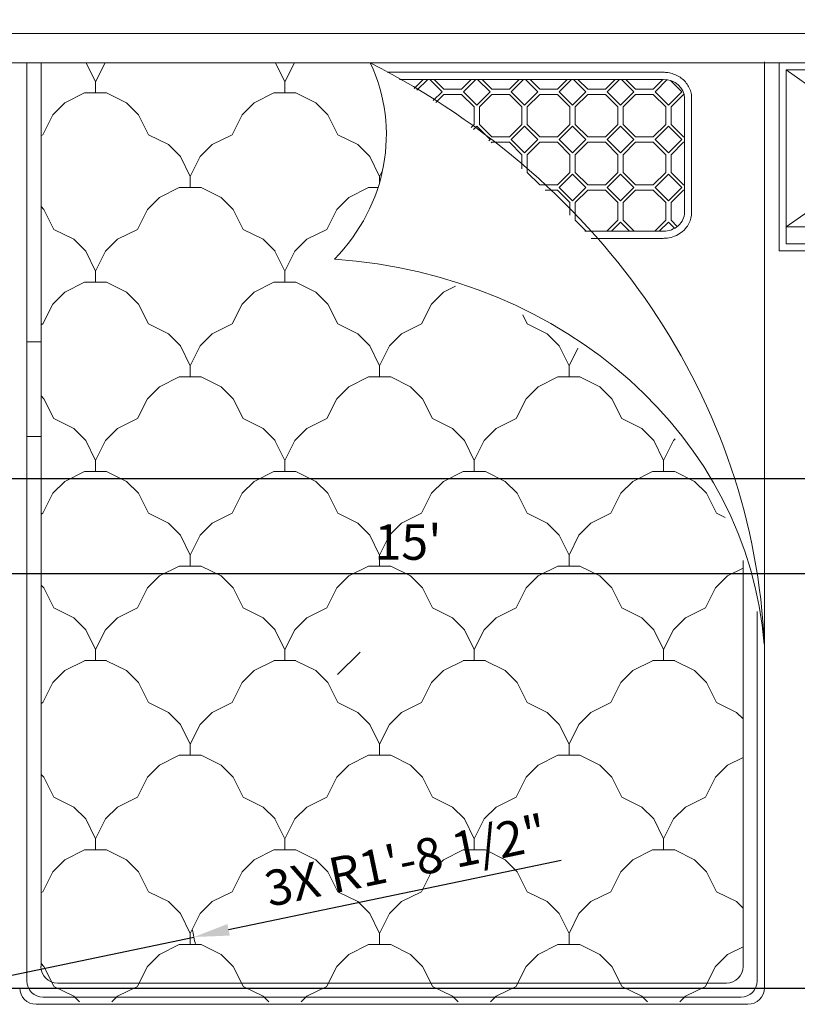
# Model space of a CAD drawing. Units: inches. Extents: x 2025 to 2528, y 1525 to 2336.
# Tile 12 of 18: x 2138 to 2192, y 2209 to 2278. Entities that reach past the tile are written whole.
import ezdxf

# ---------------------------------------------------------------- set-up
doc = ezdxf.new("R2010")
doc.units = ezdxf.units.IN
doc.layers.add('A-ANNO-DIMS', color=2, linetype='Continuous', lineweight=18)
doc.layers.add('A-FURN', color=8, linetype='Continuous', lineweight=18)
doc.styles.get("Standard").update_dxf_attribs({"font": 'arial.ttf'})
doc.dimstyles.new('Copy of ISO-25', dxfattribs={"dimtxt": 2.5, "dimasz": 2.5, "dimexe": 1.25, "dimexo": 0.625, "dimtad": 1, "dimdec": 1, "dimlunit": 4, "dimtxsty": 'Standard', "dimcen": 2.5, "dimadec": 0, "dimazin": 0, "dimtfac": 1, "dimtdec": 1, "dimtmove": 0, "dimatfit": 3, "dimfxl": 1, "dimarcsym": 0})

# ---------------------------------------------------------------- blocks, each defined once
blk = doc.blocks.new('*D6')
at = {"layer": 'A-ANNO-DIMS', "color": 0, "lineweight": -2, "transparency": 16777216}
for p, q in [((2075.013, 2282.787), (2075.013, 2237.927)), ((2255.013, 2282.787), (2255.013, 2237.927)), ((2077.513, 2239.177), (2252.513, 2239.177))]:
    blk.add_line(p, q, dxfattribs=at)
at = {"layer": 'A-ANNO-DIMS', "color": 0, "transparency": 16777216}
for points in [[(2077.513, 2239.594), (2077.513, 2238.761), (2075.013, 2239.177)], [(2252.513, 2239.594), (2252.513, 2238.761), (2255.013, 2239.177)]]:
    blk.add_solid(points, dxfattribs=at)
at = {"layer": 'Defpoints', "color": 0, "transparency": 16777216}
for p in [(2075.013, 2283.412), (2255.013, 2283.412), (2255.013, 2239.177)]:
    blk.add_point(p, dxfattribs=at)
at = {"layer": 'A-ANNO-DIMS', "color": 0, "transparency": 16777216, "insert": (2165.013, 2241.079), "char_height": 2.5, "attachment_point": 5}
blk.add_mtext("15'", dxfattribs=at)
blk = doc.blocks.new('A$C029D5C69')
for p, q in [((2.2315, 2.0693), (0.4164, 2.0693)), ((0.4164, 2.0066), (2.2315, 2.0066)), ((0.5403, 0.0502), (0.5403, 2.0066)), ((0.5706, 0.0805), (0.5706, 2.0066)), ((0.6869, 1.966), (0.6666, 2.0066)), ((0.7072, 2.0066), (0.6869, 1.966)), ((1.0902, 1.966), (1.0699, 2.0066)), ((1.1106, 2.0066), (1.0902, 1.966)), ((2.1114, 2.0087), (2.1114, 0.0351)), ((2.6479, 2.0066), (2.1429, 2.0066)), ((2.1429, 2.0066), (2.1429, 1.606)), ((1.8954, 1.9865), (1.3081, 1.9865)), ((2.6328, 1.9915), (2.158, 1.9915)), ((2.158, 1.9915), (2.158, 1.6211)), ((0.6869, 1.9425), (0.6869, 1.966)), ((0.6869, 1.9425), (0.6869, 1.966)), ((1.0902, 1.9425), (1.0902, 1.966)), ((1.0902, 1.9425), (1.0902, 1.966)), ((1.8954, 1.9713), (1.3339, 1.9713)), ((1.3849, 1.9713), (1.3656, 1.952)), ((1.3945, 1.9713), (1.3714, 1.9483)), ((1.4249, 1.945), (1.3986, 1.9713)), ((1.4288, 1.9507), (1.4081, 1.9713)), ((1.487, 1.9713), (1.4664, 1.9507)), ((1.4966, 1.9713), (1.4703, 1.945)), ((1.527, 1.945), (1.5007, 1.9713)), ((1.5309, 1.9507), (1.5102, 1.9713)), ((1.5891, 1.9713), (1.5685, 1.9507)), ((1.5987, 1.9713), (1.5724, 1.945)), ((1.6291, 1.945), (1.6028, 1.9713)), ((1.633, 1.9507), (1.6123, 1.9713)), ((1.6912, 1.9713), (1.6706, 1.9507)), ((1.7008, 1.9713), (1.6745, 1.945)), ((1.7312, 1.945), (1.7049, 1.9713)), ((1.7351, 1.9507), (1.7144, 1.9713)), ((1.7933, 1.9713), (1.7727, 1.9507)), ((1.8029, 1.9713), (1.7766, 1.945)), ((1.8333, 1.945), (1.807, 1.9713)), ((1.8372, 1.9507), (1.8165, 1.9713)), ((1.8954, 1.9713), (1.8748, 1.9507)), ((1.9043, 1.9707), (1.8787, 1.945)), ((1.9354, 1.945), (1.9114, 1.969)), ((0.6634, 1.9425), (0.621, 1.9213)), ((0.6634, 1.9425), (0.621, 1.9213)), ((0.6869, 1.9425), (0.6634, 1.9425)), ((0.6869, 1.9425), (0.7104, 1.9425)), ((0.7528, 1.9213), (0.7104, 1.9425)), ((0.7528, 1.9213), (0.7104, 1.9425)), ((1.0668, 1.9425), (1.0244, 1.9213)), ((1.0668, 1.9425), (1.0244, 1.9213)), ((1.0902, 1.9425), (1.0668, 1.9425)), ((1.0902, 1.9425), (1.1137, 1.9425)), ((1.1561, 1.9213), (1.1137, 1.9425)), ((1.1561, 1.9213), (1.1137, 1.9425)), ((1.4249, 1.945), (1.4059, 1.926)), ((1.4288, 1.9394), (1.4116, 1.9222)), ((1.4476, 1.9507), (1.4288, 1.9507)), ((1.4288, 1.9393), (1.4476, 1.9393)), ((1.4476, 1.9507), (1.4664, 1.9507)), ((1.4664, 1.9393), (1.4476, 1.9393)), ((1.493, 1.9128), (1.4664, 1.9394)), ((1.4986, 1.9167), (1.4703, 1.945)), ((1.527, 1.945), (1.4986, 1.9167)), ((1.5309, 1.9394), (1.5043, 1.9128)), ((1.5497, 1.9507), (1.5309, 1.9507)), ((1.5309, 1.9393), (1.5497, 1.9393)), ((1.5497, 1.9507), (1.5685, 1.9507)), ((1.5685, 1.9393), (1.5497, 1.9393)), ((1.595, 1.9128), (1.5685, 1.9394)), ((1.6007, 1.9167), (1.5724, 1.945)), ((1.6291, 1.945), (1.6007, 1.9167)), ((1.633, 1.9394), (1.6064, 1.9128)), ((1.6518, 1.9507), (1.633, 1.9507)), ((1.633, 1.9393), (1.6518, 1.9393)), ((1.6518, 1.9507), (1.6706, 1.9507)), ((1.6706, 1.9393), (1.6518, 1.9393)), ((1.6971, 1.9128), (1.6706, 1.9394)), ((1.7028, 1.9167), (1.6745, 1.945)), ((1.7312, 1.945), (1.7028, 1.9167)), ((1.7351, 1.9394), (1.7085, 1.9128)), ((1.7539, 1.9507), (1.7351, 1.9507)), ((1.7351, 1.9393), (1.7539, 1.9393)), ((1.7539, 1.9507), (1.7727, 1.9507)), ((1.7727, 1.9393), (1.7539, 1.9393)), ((1.7992, 1.9128), (1.7727, 1.9394)), ((1.8049, 1.9167), (1.7766, 1.945)), ((1.8333, 1.945), (1.8049, 1.9167)), ((1.8372, 1.9394), (1.8106, 1.9128)), ((1.856, 1.9507), (1.8372, 1.9507)), ((1.8372, 1.9393), (1.856, 1.9393)), ((1.856, 1.9507), (1.8748, 1.9507)), ((1.8748, 1.9393), (1.856, 1.9393)), ((1.9013, 1.9128), (1.8748, 1.9394)), ((1.907, 1.9167), (1.8787, 1.945)), ((1.9354, 1.945), (1.907, 1.9167)), ((1.9393, 1.9394), (1.9127, 1.9128)), ((1.9393, 1.9393), (1.9404, 1.9393)), ((1.9414, 1.688), (1.9414, 1.931)), ((1.9565, 1.688), (1.9565, 1.931)), ((0.621, 1.9213), (0.5955, 1.8958)), ((0.7783, 1.8958), (0.7528, 1.9213)), ((1.0243, 1.9213), (0.9988, 1.8958)), ((1.1816, 1.8958), (1.1561, 1.9213)), ((1.493, 1.8752), (1.493, 1.9128)), ((1.5043, 1.8752), (1.5043, 1.9128)), ((1.595, 1.8752), (1.595, 1.9128)), ((1.6064, 1.8752), (1.6064, 1.9128)), ((1.6971, 1.8752), (1.6971, 1.9128)), ((1.7085, 1.8752), (1.7085, 1.9128)), ((1.7992, 1.8752), (1.7992, 1.9128)), ((1.8106, 1.8752), (1.8106, 1.9128)), ((1.9013, 1.8752), (1.9013, 1.9128)), ((1.9127, 1.8752), (1.9127, 1.9128)), ((0.5955, 1.8958), (0.5743, 1.8534)), ((0.7995, 1.8534), (0.7783, 1.8958)), ((0.9989, 1.8958), (0.9777, 1.8534)), ((1.2028, 1.8534), (1.1816, 1.8958)), ((1.493, 1.8752), (1.4867, 1.869)), ((1.4986, 1.8713), (1.4922, 1.8648)), ((1.527, 1.8429), (1.4986, 1.8713)), ((1.5309, 1.8486), (1.5043, 1.8752)), ((1.595, 1.8752), (1.5685, 1.8486)), ((1.6007, 1.8713), (1.5724, 1.8429)), ((1.6291, 1.8429), (1.6007, 1.8713)), ((1.633, 1.8486), (1.6064, 1.8752)), ((1.6971, 1.8752), (1.6706, 1.8486)), ((1.7028, 1.8713), (1.6745, 1.8429)), ((1.7312, 1.8429), (1.7028, 1.8713)), ((1.7351, 1.8486), (1.7085, 1.8752)), ((1.7992, 1.8752), (1.7727, 1.8486)), ((1.8049, 1.8713), (1.7766, 1.8429)), ((1.8333, 1.8429), (1.8049, 1.8713)), ((1.8372, 1.8486), (1.8106, 1.8752)), ((1.9013, 1.8752), (1.8748, 1.8486)), ((1.907, 1.8713), (1.8787, 1.8429)), ((1.9354, 1.8429), (1.907, 1.8713)), ((1.9393, 1.8486), (1.9127, 1.8752)), ((0.5743, 1.8534), (0.5706, 1.8515)), ((0.5743, 1.8534), (0.5706, 1.8515)), ((0.8419, 1.8322), (0.7995, 1.8534)), ((0.8419, 1.8322), (0.7995, 1.8534)), ((0.9777, 1.8534), (0.9353, 1.8322)), ((0.9777, 1.8534), (0.9353, 1.8322)), ((1.2452, 1.8322), (1.2028, 1.8534)), ((1.2452, 1.8322), (1.2028, 1.8534)), ((1.5497, 1.8486), (1.5309, 1.8486)), ((1.5497, 1.8486), (1.5685, 1.8486)), ((1.6518, 1.8486), (1.633, 1.8486)), ((1.6518, 1.8486), (1.6706, 1.8486)), ((1.7539, 1.8486), (1.7351, 1.8486)), ((1.7539, 1.8486), (1.7727, 1.8486)), ((1.856, 1.8486), (1.8372, 1.8486)), ((1.856, 1.8486), (1.8748, 1.8486)), ((1.9414, 1.8486), (1.9393, 1.8486)), ((0.8674, 1.8067), (0.8419, 1.8322)), ((0.9352, 1.8322), (0.9097, 1.8067)), ((1.2707, 1.8067), (1.2452, 1.8322)), ((1.527, 1.8429), (1.5242, 1.8401)), ((1.5309, 1.8373), (1.5295, 1.8359)), ((1.5309, 1.8373), (1.5497, 1.8373)), ((1.5685, 1.8373), (1.5497, 1.8373)), ((1.595, 1.8107), (1.5685, 1.8373)), ((1.6007, 1.8146), (1.5724, 1.8429)), ((1.6291, 1.8429), (1.6007, 1.8146)), ((1.633, 1.8373), (1.6064, 1.8107)), ((1.633, 1.8373), (1.6518, 1.8373)), ((1.6706, 1.8373), (1.6518, 1.8373)), ((1.6971, 1.8107), (1.6706, 1.8373)), ((1.7028, 1.8146), (1.6745, 1.8429)), ((1.7312, 1.8429), (1.7028, 1.8146)), ((1.7351, 1.8373), (1.7085, 1.8107)), ((1.7351, 1.8373), (1.7539, 1.8373)), ((1.7727, 1.8373), (1.7539, 1.8373)), ((1.7992, 1.8107), (1.7727, 1.8373)), ((1.8049, 1.8146), (1.7766, 1.8429)), ((1.8333, 1.8429), (1.8049, 1.8146)), ((1.8372, 1.8373), (1.8106, 1.8107)), ((1.8372, 1.8373), (1.856, 1.8373)), ((1.8748, 1.8373), (1.856, 1.8373)), ((1.9013, 1.8107), (1.8748, 1.8373)), ((1.907, 1.8146), (1.8787, 1.8429)), ((1.9354, 1.8429), (1.907, 1.8146)), ((1.9393, 1.8373), (1.9127, 1.8107)), ((1.9393, 1.8373), (1.9414, 1.8373)), ((0.8886, 1.7643), (0.8674, 1.8067)), ((0.9098, 1.8067), (0.8886, 1.7643)), ((1.2919, 1.7643), (1.2707, 1.8067)), ((1.595, 1.7806), (1.595, 1.8107)), ((1.6064, 1.7731), (1.6064, 1.8107)), ((1.6971, 1.7731), (1.6971, 1.8107)), ((1.7085, 1.7731), (1.7085, 1.8107)), ((1.7992, 1.7731), (1.7992, 1.8107)), ((1.8106, 1.7731), (1.8106, 1.8107)), ((1.9013, 1.7731), (1.9013, 1.8107)), ((1.9127, 1.7731), (1.9127, 1.8107)), ((0.8886, 1.7408), (0.8886, 1.7643)), ((1.2981, 1.7768), (1.2919, 1.7643)), ((1.2919, 1.7519), (1.2919, 1.7643)), ((1.633, 1.7465), (1.6064, 1.7731)), ((1.6971, 1.7731), (1.6706, 1.7465)), ((1.7028, 1.7692), (1.6745, 1.7408)), ((1.7312, 1.7408), (1.7028, 1.7692)), ((1.7351, 1.7465), (1.7085, 1.7731)), ((1.7992, 1.7731), (1.7727, 1.7465)), ((1.8049, 1.7692), (1.7766, 1.7408)), ((1.8333, 1.7408), (1.8049, 1.7692)), ((1.8372, 1.7465), (1.8106, 1.7731)), ((1.9013, 1.7731), (1.8748, 1.7465)), ((1.907, 1.7692), (1.8787, 1.7408)), ((1.9354, 1.7408), (1.907, 1.7692)), ((1.9393, 1.7465), (1.9127, 1.7731)), ((1.6518, 1.7465), (1.633, 1.7465)), ((1.6518, 1.7465), (1.6706, 1.7465)), ((1.7539, 1.7465), (1.7351, 1.7465)), ((1.7539, 1.7465), (1.7727, 1.7465)), ((1.856, 1.7465), (1.8372, 1.7465)), ((1.856, 1.7465), (1.8748, 1.7465)), ((1.9414, 1.7465), (1.9393, 1.7465)), ((0.8651, 1.7408), (0.8227, 1.7196)), ((0.8651, 1.7408), (0.8227, 1.7196)), ((0.912, 1.7408), (0.8651, 1.7408)), ((0.9544, 1.7196), (0.912, 1.7408)), ((0.9544, 1.7196), (0.912, 1.7408)), ((1.2684, 1.7408), (1.226, 1.7196)), ((1.2684, 1.7408), (1.226, 1.7196)), ((1.2885, 1.7408), (1.2684, 1.7408)), ((1.6443, 1.7352), (1.6518, 1.7352)), ((1.6706, 1.7352), (1.6518, 1.7352)), ((1.6971, 1.7086), (1.6706, 1.7352)), ((1.7028, 1.7125), (1.6745, 1.7408)), ((1.7312, 1.7408), (1.7028, 1.7125)), ((1.7351, 1.7352), (1.7085, 1.7086)), ((1.7351, 1.7352), (1.7539, 1.7352)), ((1.7727, 1.7352), (1.7539, 1.7352)), ((1.7992, 1.7086), (1.7727, 1.7352)), ((1.8049, 1.7125), (1.7766, 1.7408)), ((1.8333, 1.7408), (1.8049, 1.7125)), ((1.8372, 1.7352), (1.8106, 1.7086)), ((1.8372, 1.7352), (1.856, 1.7352)), ((1.8748, 1.7352), (1.856, 1.7352)), ((1.9013, 1.7086), (1.8748, 1.7352)), ((1.907, 1.7125), (1.8787, 1.7408)), ((1.9354, 1.7408), (1.907, 1.7125)), ((1.9393, 1.7352), (1.9127, 1.7086)), ((1.9393, 1.7352), (1.9414, 1.7352)), ((0.5766, 1.6941), (0.5706, 1.7002)), ((0.8227, 1.7196), (0.7972, 1.6941)), ((0.98, 1.6941), (0.9545, 1.7196)), ((1.226, 1.7196), (1.2005, 1.6941)), ((1.6971, 1.682), (1.6971, 1.7086)), ((1.7085, 1.671), (1.7085, 1.7086)), ((1.7992, 1.671), (1.7992, 1.7086)), ((1.8106, 1.671), (1.8106, 1.7086)), ((1.9013, 1.671), (1.9013, 1.7086)), ((1.9127, 1.671), (1.9127, 1.7086)), ((0.5978, 1.6517), (0.5766, 1.6941)), ((0.7972, 1.6941), (0.776, 1.6517)), ((1.0011, 1.6517), (0.9799, 1.6941)), ((1.2005, 1.6941), (1.1793, 1.6517)), ((1.7318, 1.6477), (1.7085, 1.671)), ((1.7992, 1.671), (1.7759, 1.6477)), ((1.8049, 1.6671), (1.7855, 1.6477)), ((1.8244, 1.6477), (1.8049, 1.6671)), ((1.8339, 1.6477), (1.8106, 1.671)), ((1.9013, 1.671), (1.878, 1.6477)), ((1.907, 1.6671), (1.8876, 1.6477)), ((1.9202, 1.6539), (1.907, 1.6671)), ((1.926, 1.6577), (1.9127, 1.671)), ((0.6402, 1.6305), (0.5978, 1.6517)), ((0.6402, 1.6305), (0.5978, 1.6517)), ((0.776, 1.6517), (0.7336, 1.6305)), ((0.776, 1.6517), (0.7336, 1.6305)), ((1.0435, 1.6305), (1.0011, 1.6517)), ((1.0435, 1.6305), (1.0011, 1.6517)), ((1.1793, 1.6517), (1.1369, 1.6305)), ((1.1793, 1.6517), (1.1369, 1.6305)), ((1.8961, 1.6477), (1.7289, 1.6477)), ((0.6657, 1.605), (0.6402, 1.6305)), ((0.7336, 1.6305), (0.7081, 1.605)), ((1.0691, 1.605), (1.0436, 1.6305)), ((1.1369, 1.6305), (1.1114, 1.605)), ((1.8961, 1.6325), (1.7422, 1.6325)), ((2.158, 1.6211), (2.6328, 1.6211)), ((0.6869, 1.5626), (0.6657, 1.605)), ((0.7081, 1.605), (0.6869, 1.5626)), ((1.0902, 1.5626), (1.069, 1.605)), ((1.1114, 1.605), (1.0902, 1.5626)), ((2.1429, 1.606), (2.6479, 1.606)), ((0.6869, 1.5392), (0.6869, 1.5626)), ((0.6869, 1.5392), (0.6869, 1.5626)), ((1.0902, 1.5392), (1.0902, 1.5626)), ((1.0902, 1.5392), (1.0902, 1.5626)), ((0.6634, 1.5391), (0.621, 1.5179)), ((0.6634, 1.5391), (0.621, 1.5179)), ((0.6869, 1.5392), (0.6634, 1.5392)), ((0.6869, 1.5392), (0.7104, 1.5392)), ((0.7528, 1.5179), (0.7104, 1.5391)), ((0.7528, 1.5179), (0.7104, 1.5391)), ((1.0668, 1.5391), (1.0244, 1.5179)), ((1.0668, 1.5391), (1.0244, 1.5179)), ((1.0902, 1.5392), (1.0668, 1.5392)), ((1.0902, 1.5392), (1.1137, 1.5392)), ((1.1561, 1.5179), (1.1137, 1.5391)), ((1.1561, 1.5179), (1.1137, 1.5391)), ((0.621, 1.5179), (0.5955, 1.4924)), ((0.7783, 1.4924), (0.7528, 1.5179)), ((1.0243, 1.5179), (0.9988, 1.4924)), ((1.1816, 1.4924), (1.1561, 1.5179)), ((1.4277, 1.5179), (1.4022, 1.4924)), ((1.4534, 1.5308), (1.4277, 1.5179)), ((1.4534, 1.5308), (1.4277, 1.5179)), ((0.5955, 1.4925), (0.5743, 1.4501)), ((0.7995, 1.4501), (0.7783, 1.4925)), ((0.9989, 1.4925), (0.9777, 1.4501)), ((1.2028, 1.4501), (1.1816, 1.4925)), ((1.4022, 1.4925), (1.381, 1.4501)), ((1.6062, 1.4501), (1.5966, 1.4692)), ((0.5743, 1.45), (0.5706, 1.4481)), ((0.5743, 1.45), (0.5706, 1.4481)), ((0.8419, 1.4288), (0.7995, 1.45)), ((0.8419, 1.4288), (0.7995, 1.45)), ((0.9777, 1.45), (0.9353, 1.4288)), ((0.9777, 1.45), (0.9353, 1.4288)), ((1.2452, 1.4288), (1.2028, 1.45)), ((1.2452, 1.4288), (1.2028, 1.45)), ((1.381, 1.45), (1.3386, 1.4288)), ((1.381, 1.45), (1.3386, 1.4288)), ((1.6486, 1.4288), (1.6062, 1.45)), ((1.6486, 1.4288), (1.6062, 1.45)), ((0.8674, 1.4033), (0.8419, 1.4288)), ((0.9352, 1.4288), (0.9097, 1.4033)), ((1.2707, 1.4033), (1.2452, 1.4288)), ((1.3386, 1.4288), (1.3131, 1.4033)), ((1.6741, 1.4033), (1.6486, 1.4288)), ((0.5403, 1.4117), (0.5706, 1.4117)), ((0.8886, 1.361), (0.8674, 1.4034)), ((0.9098, 1.4034), (0.8886, 1.361)), ((1.2919, 1.361), (1.2707, 1.4034)), ((1.3131, 1.4034), (1.2919, 1.361)), ((1.6953, 1.361), (1.6741, 1.4034)), ((1.714, 1.3984), (1.6953, 1.361)), ((0.8886, 1.3375), (0.8886, 1.3609)), ((1.2919, 1.3375), (1.2919, 1.3609)), ((1.6953, 1.3375), (1.6953, 1.3609)), ((0.8651, 1.3374), (0.8227, 1.3162)), ((0.8651, 1.3374), (0.8227, 1.3162)), ((0.912, 1.3375), (0.8651, 1.3375)), ((0.9544, 1.3162), (0.912, 1.3374)), ((0.9544, 1.3162), (0.912, 1.3374)), ((1.2684, 1.3374), (1.226, 1.3162)), ((1.2684, 1.3374), (1.226, 1.3162)), ((1.3154, 1.3375), (1.2684, 1.3375)), ((1.3578, 1.3162), (1.3154, 1.3374)), ((1.3578, 1.3162), (1.3154, 1.3374)), ((1.6718, 1.3374), (1.6294, 1.3162)), ((1.6718, 1.3374), (1.6294, 1.3162)), ((1.7187, 1.3375), (1.6718, 1.3375)), ((1.7611, 1.3162), (1.7187, 1.3374)), ((1.7611, 1.3162), (1.7187, 1.3374)), ((0.8227, 1.3163), (0.7972, 1.2908)), ((0.98, 1.2908), (0.9545, 1.3163)), ((1.226, 1.3163), (1.2005, 1.2908)), ((1.3833, 1.2908), (1.3578, 1.3163)), ((1.6294, 1.3163), (1.6039, 1.2908)), ((1.7867, 1.2908), (1.7611, 1.3163)), ((0.5766, 1.2908), (0.5706, 1.2968)), ((0.5978, 1.2484), (0.5766, 1.2908)), ((0.7972, 1.2908), (0.776, 1.2484)), ((1.0011, 1.2484), (0.9799, 1.2908)), ((1.2005, 1.2908), (1.1793, 1.2484)), ((1.4045, 1.2484), (1.3833, 1.2908)), ((1.6039, 1.2908), (1.5827, 1.2484)), ((1.8078, 1.2484), (1.7866, 1.2908)), ((0.6402, 1.2271), (0.5978, 1.2483)), ((0.6402, 1.2271), (0.5978, 1.2483)), ((0.776, 1.2483), (0.7336, 1.2271)), ((0.776, 1.2483), (0.7336, 1.2271)), ((1.0435, 1.2271), (1.0011, 1.2483)), ((1.0435, 1.2271), (1.0011, 1.2483)), ((1.1793, 1.2483), (1.1369, 1.2271)), ((1.1793, 1.2483), (1.1369, 1.2271)), ((1.4469, 1.2271), (1.4045, 1.2483)), ((1.4469, 1.2271), (1.4045, 1.2483)), ((1.5827, 1.2483), (1.5403, 1.2271)), ((1.5827, 1.2483), (1.5403, 1.2271)), ((1.8502, 1.2271), (1.8078, 1.2483)), ((1.8502, 1.2271), (1.8078, 1.2483)), ((0.6657, 1.2017), (0.6402, 1.2272)), ((0.7336, 1.2272), (0.7081, 1.2017)), ((1.0691, 1.2017), (1.0436, 1.2272)), ((1.1369, 1.2272), (1.1114, 1.2017)), ((1.4724, 1.2017), (1.4469, 1.2272)), ((1.5403, 1.2272), (1.5148, 1.2017)), ((1.8758, 1.2017), (1.8503, 1.2272)), ((0.5403, 1.21), (0.5706, 1.21)), ((0.6869, 1.1593), (0.6657, 1.2017)), ((0.7081, 1.2017), (0.6869, 1.1593)), ((1.0902, 1.1593), (1.069, 1.2017)), ((1.1114, 1.2017), (1.0902, 1.1593)), ((1.4936, 1.1593), (1.4724, 1.2017)), ((1.5148, 1.2017), (1.4936, 1.1593)), ((1.8969, 1.1593), (1.8757, 1.2017)), ((1.9181, 1.2017), (1.8969, 1.1593)), ((1.9215, 1.2051), (1.9181, 1.2017)), ((0.6869, 1.1358), (0.6869, 1.1593)), ((0.6869, 1.1358), (0.6869, 1.1593)), ((1.0902, 1.1358), (1.0902, 1.1593)), ((1.0902, 1.1358), (1.0902, 1.1593)), ((1.4936, 1.1358), (1.4936, 1.1593)), ((1.4936, 1.1358), (1.4936, 1.1593)), ((1.8969, 1.1358), (1.8969, 1.1593)), ((1.8969, 1.1358), (1.8969, 1.1593)), ((0.6634, 1.1358), (0.621, 1.1146)), ((0.6634, 1.1358), (0.621, 1.1146)), ((0.6869, 1.1358), (0.6634, 1.1358)), ((0.6869, 1.1358), (0.7104, 1.1358)), ((0.7528, 1.1146), (0.7104, 1.1358)), ((0.7528, 1.1146), (0.7104, 1.1358)), ((1.0668, 1.1358), (1.0244, 1.1146)), ((1.0668, 1.1358), (1.0244, 1.1146)), ((1.0902, 1.1358), (1.0668, 1.1358)), ((1.0902, 1.1358), (1.1137, 1.1358)), ((1.1561, 1.1146), (1.1137, 1.1358)), ((1.1561, 1.1146), (1.1137, 1.1358)), ((1.4701, 1.1358), (1.4277, 1.1146)), ((1.4701, 1.1358), (1.4277, 1.1146)), ((1.4936, 1.1358), (1.4701, 1.1358)), ((1.4936, 1.1358), (1.5171, 1.1358)), ((1.5595, 1.1146), (1.5171, 1.1358)), ((1.5595, 1.1146), (1.5171, 1.1358)), ((1.8735, 1.1358), (1.8311, 1.1146)), ((1.8735, 1.1358), (1.8311, 1.1146)), ((1.8969, 1.1358), (1.8735, 1.1358)), ((1.8969, 1.1358), (1.9204, 1.1358)), ((1.9628, 1.1146), (1.9204, 1.1358)), ((1.9628, 1.1146), (1.9204, 1.1358)), ((0.621, 1.1146), (0.5955, 1.0891)), ((0.7783, 1.0891), (0.7528, 1.1146)), ((1.0243, 1.1146), (0.9988, 1.0891)), ((1.1816, 1.0891), (1.1561, 1.1146)), ((1.4277, 1.1146), (1.4022, 1.0891)), ((1.585, 1.0891), (1.5595, 1.1146)), ((1.831, 1.1146), (1.8055, 1.0891)), ((1.9883, 1.0891), (1.9628, 1.1146)), ((0.5955, 1.0891), (0.5743, 1.0467)), ((0.7995, 1.0467), (0.7783, 1.0891)), ((0.9989, 1.0891), (0.9777, 1.0467)), ((1.2028, 1.0467), (1.1816, 1.0891)), ((1.4022, 1.0891), (1.381, 1.0467)), ((1.6062, 1.0467), (1.585, 1.0891)), ((1.8056, 1.0891), (1.7844, 1.0467)), ((2.0095, 1.0467), (1.9883, 1.0891)), ((0.5743, 1.0467), (0.5706, 1.0448)), ((0.5743, 1.0467), (0.5706, 1.0448)), ((0.8419, 1.0255), (0.7995, 1.0467)), ((0.8419, 1.0255), (0.7995, 1.0467)), ((0.9777, 1.0467), (0.9353, 1.0255)), ((0.9777, 1.0467), (0.9353, 1.0255)), ((1.2452, 1.0255), (1.2028, 1.0467)), ((1.2452, 1.0255), (1.2028, 1.0467)), ((1.381, 1.0467), (1.3386, 1.0255)), ((1.381, 1.0467), (1.3386, 1.0255)), ((1.6486, 1.0255), (1.6062, 1.0467)), ((1.6486, 1.0255), (1.6062, 1.0467)), ((1.7844, 1.0467), (1.742, 1.0255)), ((1.7844, 1.0467), (1.742, 1.0255)), ((2.0276, 1.0376), (2.0095, 1.0467)), ((2.0276, 1.0376), (2.0095, 1.0467)), ((0.8674, 1), (0.8419, 1.0255)), ((0.9352, 1.0255), (0.9097, 1)), ((1.2707, 1), (1.2452, 1.0255)), ((1.3386, 1.0255), (1.3131, 1)), ((1.6741, 1), (1.6486, 1.0255)), ((1.7419, 1.0255), (1.7164, 1)), ((0.8886, 0.9576), (0.8674, 1)), ((0.9098, 1), (0.8886, 0.9576)), ((1.2919, 0.9576), (1.2707, 1)), ((1.3131, 1), (1.2919, 0.9576)), ((1.6953, 0.9576), (1.6741, 1)), ((1.7165, 1), (1.6953, 0.9576)), ((0.8886, 0.9341), (0.8886, 0.9576)), ((1.2919, 0.9341), (1.2919, 0.9576)), ((1.6953, 0.9341), (1.6953, 0.9576)), ((2.066, 0.9457), (2.066, 0.0805)), ((0.8651, 0.9341), (0.8227, 0.9129)), ((0.8651, 0.9341), (0.8227, 0.9129)), ((0.912, 0.9341), (0.8651, 0.9341)), ((0.9544, 0.9129), (0.912, 0.9341)), ((0.9544, 0.9129), (0.912, 0.9341)), ((1.2684, 0.9341), (1.226, 0.9129)), ((1.2684, 0.9341), (1.226, 0.9129)), ((1.3154, 0.9341), (1.2684, 0.9341)), ((1.3578, 0.9129), (1.3154, 0.9341)), ((1.3578, 0.9129), (1.3154, 0.9341)), ((1.6718, 0.9341), (1.6294, 0.9129)), ((1.6718, 0.9341), (1.6294, 0.9129)), ((1.7187, 0.9341), (1.6718, 0.9341)), ((1.7611, 0.9129), (1.7187, 0.9341)), ((1.7611, 0.9129), (1.7187, 0.9341)), ((2.066, 0.9295), (2.0327, 0.9129)), ((2.066, 0.9295), (2.0327, 0.9129)), ((0.8227, 0.9129), (0.7972, 0.8874)), ((0.98, 0.8874), (0.9545, 0.9129)), ((1.226, 0.9129), (1.2005, 0.8874)), ((1.3833, 0.8874), (1.3578, 0.9129)), ((1.6294, 0.9129), (1.6039, 0.8874)), ((1.7867, 0.8874), (1.7611, 0.9129)), ((2.0327, 0.9129), (2.0072, 0.8874)), ((0.5766, 0.8874), (0.5706, 0.8935)), ((0.5978, 0.845), (0.5766, 0.8874)), ((0.7972, 0.8874), (0.776, 0.845)), ((1.0011, 0.845), (0.9799, 0.8874)), ((1.2005, 0.8874), (1.1793, 0.845)), ((1.4045, 0.845), (1.3833, 0.8874)), ((1.6039, 0.8874), (1.5827, 0.845)), ((1.8078, 0.845), (1.7866, 0.8874)), ((2.0072, 0.8874), (1.986, 0.845)), ((0.6402, 0.8238), (0.5978, 0.845)), ((0.6402, 0.8238), (0.5978, 0.845)), ((0.776, 0.845), (0.7336, 0.8238)), ((0.776, 0.845), (0.7336, 0.8238)), ((1.0435, 0.8238), (1.0011, 0.845)), ((1.0435, 0.8238), (1.0011, 0.845)), ((1.1793, 0.845), (1.1369, 0.8238)), ((1.1793, 0.845), (1.1369, 0.8238)), ((1.4469, 0.8238), (1.4045, 0.845)), ((1.4469, 0.8238), (1.4045, 0.845)), ((1.5827, 0.845), (1.5403, 0.8238)), ((1.5827, 0.845), (1.5403, 0.8238)), ((1.8502, 0.8238), (1.8078, 0.845)), ((1.8502, 0.8238), (1.8078, 0.845)), ((1.986, 0.845), (1.9436, 0.8238)), ((1.986, 0.845), (1.9436, 0.8238)), ((0.6657, 0.7983), (0.6402, 0.8238)), ((0.7336, 0.8238), (0.7081, 0.7983)), ((1.0691, 0.7983), (1.0436, 0.8238)), ((1.1369, 0.8238), (1.1114, 0.7983)), ((1.4724, 0.7983), (1.4469, 0.8238)), ((1.5403, 0.8238), (1.5148, 0.7983)), ((1.8758, 0.7983), (1.8503, 0.8238)), ((1.9436, 0.8238), (1.9181, 0.7983)), ((2.0962, 0.8369), (2.0962, 0.0502)), ((0.6869, 0.7559), (0.6657, 0.7983)), ((0.7081, 0.7983), (0.6869, 0.7559)), ((1.0902, 0.7559), (1.069, 0.7983)), ((1.1114, 0.7983), (1.0902, 0.7559)), ((1.4936, 0.7559), (1.4724, 0.7983)), ((1.5148, 0.7983), (1.4936, 0.7559)), ((1.8969, 0.7559), (1.8757, 0.7983)), ((1.9181, 0.7983), (1.8969, 0.7559)), ((0.6869, 0.7325), (0.6869, 0.7559)), ((0.6869, 0.7325), (0.6869, 0.7559)), ((1.0902, 0.7325), (1.0902, 0.7559)), ((1.0902, 0.7325), (1.0902, 0.7559)), ((1.4936, 0.7325), (1.4936, 0.7559)), ((1.4936, 0.7325), (1.4936, 0.7559)), ((1.8969, 0.7325), (1.8969, 0.7559)), ((1.8969, 0.7325), (1.8969, 0.7559)), ((1.2024, 0.7028), (1.2503, 0.7507)), ((0.6634, 0.7324), (0.621, 0.7112)), ((0.6634, 0.7324), (0.621, 0.7112)), ((0.6869, 0.7325), (0.6634, 0.7325)), ((0.6869, 0.7325), (0.7104, 0.7325)), ((0.7528, 0.7112), (0.7104, 0.7324)), ((0.7528, 0.7112), (0.7104, 0.7324)), ((1.0668, 0.7324), (1.0244, 0.7112)), ((1.0668, 0.7324), (1.0244, 0.7112)), ((1.0902, 0.7325), (1.0668, 0.7325)), ((1.0902, 0.7325), (1.1137, 0.7325)), ((1.1561, 0.7112), (1.1137, 0.7324)), ((1.1561, 0.7112), (1.1137, 0.7324)), ((1.4701, 0.7324), (1.4277, 0.7112)), ((1.4701, 0.7324), (1.4277, 0.7112)), ((1.4936, 0.7325), (1.4701, 0.7325)), ((1.4936, 0.7325), (1.5171, 0.7325)), ((1.5595, 0.7112), (1.5171, 0.7324)), ((1.5595, 0.7112), (1.5171, 0.7324)), ((1.8735, 0.7324), (1.8311, 0.7112)), ((1.8735, 0.7324), (1.8311, 0.7112)), ((1.8969, 0.7325), (1.8735, 0.7325)), ((1.8969, 0.7325), (1.9204, 0.7325)), ((1.9628, 0.7112), (1.9204, 0.7324)), ((1.9628, 0.7112), (1.9204, 0.7324)), ((0.621, 0.7113), (0.5955, 0.6858)), ((0.7783, 0.6858), (0.7528, 0.7113)), ((1.0243, 0.7113), (0.9988, 0.6858)), ((1.1816, 0.6858), (1.1561, 0.7113)), ((1.4277, 0.7113), (1.4022, 0.6858)), ((1.585, 0.6858), (1.5595, 0.7113)), ((1.831, 0.7113), (1.8055, 0.6858)), ((1.9883, 0.6858), (1.9628, 0.7113)), ((0.5955, 0.6858), (0.5743, 0.6434)), ((0.7995, 0.6434), (0.7783, 0.6858)), ((0.9989, 0.6858), (0.9777, 0.6434)), ((1.2028, 0.6434), (1.1816, 0.6858)), ((1.4022, 0.6858), (1.381, 0.6434)), ((1.6062, 0.6434), (1.585, 0.6858)), ((1.8056, 0.6858), (1.7844, 0.6434)), ((2.0095, 0.6434), (1.9883, 0.6858)), ((0.5743, 0.6433), (0.5706, 0.6414)), ((0.5743, 0.6433), (0.5706, 0.6414)), ((0.8419, 0.6221), (0.7995, 0.6433)), ((0.8419, 0.6221), (0.7995, 0.6433)), ((0.9777, 0.6433), (0.9353, 0.6221)), ((0.9777, 0.6433), (0.9353, 0.6221)), ((1.2452, 0.6221), (1.2028, 0.6433)), ((1.2452, 0.6221), (1.2028, 0.6433)), ((1.381, 0.6433), (1.3386, 0.6221)), ((1.381, 0.6433), (1.3386, 0.6221)), ((1.6486, 0.6221), (1.6062, 0.6433)), ((1.6486, 0.6221), (1.6062, 0.6433)), ((1.7844, 0.6433), (1.742, 0.6221)), ((1.7844, 0.6433), (1.742, 0.6221)), ((2.0519, 0.6221), (2.0095, 0.6433)), ((2.0519, 0.6221), (2.0095, 0.6433)), ((0.8674, 0.5967), (0.8419, 0.6222)), ((0.9352, 0.6222), (0.9097, 0.5967)), ((1.2707, 0.5967), (1.2452, 0.6222)), ((1.3386, 0.6222), (1.3131, 0.5967)), ((1.6741, 0.5967), (1.6486, 0.6222)), ((1.7419, 0.6222), (1.7164, 0.5967)), ((2.066, 0.6081), (2.0519, 0.6222)), ((0.8886, 0.5543), (0.8674, 0.5967)), ((0.9098, 0.5967), (0.8886, 0.5543)), ((1.2919, 0.5543), (1.2707, 0.5967)), ((1.3131, 0.5967), (1.2919, 0.5543)), ((1.6953, 0.5543), (1.6741, 0.5967)), ((1.7165, 0.5967), (1.6953, 0.5543)), ((0.8886, 0.5308), (0.8886, 0.5543)), ((1.2919, 0.5308), (1.2919, 0.5543)), ((1.6953, 0.5308), (1.6953, 0.5543)), ((0.8651, 0.5308), (0.8227, 0.5096)), ((0.8651, 0.5308), (0.8227, 0.5096)), ((0.912, 0.5308), (0.8651, 0.5308)), ((0.9544, 0.5096), (0.912, 0.5308)), ((0.9544, 0.5096), (0.912, 0.5308)), ((1.2684, 0.5308), (1.226, 0.5096)), ((1.2684, 0.5308), (1.226, 0.5096)), ((1.3154, 0.5308), (1.2684, 0.5308)), ((1.3578, 0.5096), (1.3154, 0.5308)), ((1.3578, 0.5096), (1.3154, 0.5308)), ((1.6718, 0.5308), (1.6294, 0.5096)), ((1.6718, 0.5308), (1.6294, 0.5096)), ((1.7187, 0.5308), (1.6718, 0.5308)), ((1.7611, 0.5096), (1.7187, 0.5308)), ((1.7611, 0.5096), (1.7187, 0.5308)), ((2.066, 0.5262), (2.0327, 0.5096)), ((2.066, 0.5262), (2.0327, 0.5096)), ((0.8227, 0.5096), (0.7972, 0.4841)), ((0.98, 0.4841), (0.9545, 0.5096)), ((1.226, 0.5096), (1.2005, 0.4841)), ((1.3833, 0.4841), (1.3578, 0.5096)), ((1.6294, 0.5096), (1.6039, 0.4841)), ((1.7867, 0.4841), (1.7611, 0.5096)), ((2.0327, 0.5096), (2.0072, 0.4841)), ((0.5766, 0.4841), (0.5706, 0.4901)), ((0.5978, 0.4417), (0.5766, 0.4841)), ((0.7972, 0.4841), (0.776, 0.4417)), ((1.0011, 0.4417), (0.9799, 0.4841)), ((1.2005, 0.4841), (1.1793, 0.4417)), ((1.4045, 0.4417), (1.3833, 0.4841)), ((1.6039, 0.4841), (1.5827, 0.4417)), ((1.8078, 0.4417), (1.7866, 0.4841)), ((2.0072, 0.4841), (1.986, 0.4417)), ((0.6402, 0.4205), (0.5978, 0.4417)), ((0.6402, 0.4205), (0.5978, 0.4417)), ((0.776, 0.4417), (0.7336, 0.4205)), ((0.776, 0.4417), (0.7336, 0.4205)), ((1.0435, 0.4205), (1.0011, 0.4417)), ((1.0435, 0.4205), (1.0011, 0.4417)), ((1.1793, 0.4417), (1.1369, 0.4205)), ((1.1793, 0.4417), (1.1369, 0.4205)), ((1.4469, 0.4205), (1.4045, 0.4417)), ((1.4469, 0.4205), (1.4045, 0.4417)), ((1.5827, 0.4417), (1.5403, 0.4205)), ((1.5827, 0.4417), (1.5403, 0.4205)), ((1.8502, 0.4205), (1.8078, 0.4417)), ((1.8502, 0.4205), (1.8078, 0.4417)), ((1.986, 0.4417), (1.9436, 0.4205)), ((1.986, 0.4417), (1.9436, 0.4205)), ((0.6657, 0.395), (0.6402, 0.4205)), ((0.7336, 0.4205), (0.7081, 0.395)), ((1.0691, 0.395), (1.0436, 0.4205)), ((1.1369, 0.4205), (1.1114, 0.395)), ((1.4724, 0.395), (1.4469, 0.4205)), ((1.5403, 0.4205), (1.5148, 0.395)), ((1.8758, 0.395), (1.8503, 0.4205)), ((1.9436, 0.4205), (1.9181, 0.395)), ((0.6869, 0.3526), (0.6657, 0.395)), ((0.7081, 0.395), (0.6869, 0.3526)), ((1.0902, 0.3526), (1.069, 0.395)), ((1.1114, 0.395), (1.0902, 0.3526)), ((1.4936, 0.3526), (1.4724, 0.395)), ((1.5148, 0.395), (1.4936, 0.3526)), ((1.8969, 0.3526), (1.8757, 0.395)), ((1.9181, 0.395), (1.8969, 0.3526)), ((0.6869, 0.3291), (0.6869, 0.3526)), ((0.6869, 0.3291), (0.6869, 0.3526)), ((1.0902, 0.3291), (1.0902, 0.3526)), ((1.0902, 0.3291), (1.0902, 0.3526)), ((1.4936, 0.3291), (1.4936, 0.3526)), ((1.4936, 0.3291), (1.4936, 0.3526)), ((1.8969, 0.3291), (1.8969, 0.3526)), ((1.8969, 0.3291), (1.8969, 0.3526)), ((0.6634, 0.3291), (0.621, 0.3079)), ((0.6634, 0.3291), (0.621, 0.3079)), ((0.6869, 0.3291), (0.6634, 0.3291)), ((0.6869, 0.3291), (0.7104, 0.3291)), ((0.7528, 0.3079), (0.7104, 0.3291)), ((0.7528, 0.3079), (0.7104, 0.3291)), ((1.0668, 0.3291), (1.0244, 0.3079)), ((1.0668, 0.3291), (1.0244, 0.3079)), ((1.0902, 0.3291), (1.0668, 0.3291)), ((1.0902, 0.3291), (1.1137, 0.3291)), ((1.1561, 0.3079), (1.1137, 0.3291)), ((1.1561, 0.3079), (1.1137, 0.3291)), ((1.4701, 0.3291), (1.4277, 0.3079)), ((1.4701, 0.3291), (1.4277, 0.3079)), ((1.4936, 0.3291), (1.4701, 0.3291)), ((1.4936, 0.3291), (1.5171, 0.3291)), ((1.5595, 0.3079), (1.5171, 0.3291)), ((1.5595, 0.3079), (1.5171, 0.3291)), ((1.8735, 0.3291), (1.8311, 0.3079)), ((1.8735, 0.3291), (1.8311, 0.3079)), ((1.8969, 0.3291), (1.8735, 0.3291)), ((1.8969, 0.3291), (1.9204, 0.3291)), ((1.9628, 0.3079), (1.9204, 0.3291)), ((1.9628, 0.3079), (1.9204, 0.3291)), ((0.621, 0.3079), (0.5955, 0.2824)), ((0.7783, 0.2824), (0.7528, 0.3079)), ((1.0243, 0.3079), (0.9988, 0.2824)), ((1.1816, 0.2824), (1.1561, 0.3079)), ((1.4277, 0.3079), (1.4022, 0.2824)), ((1.585, 0.2824), (1.5595, 0.3079)), ((1.831, 0.3079), (1.8055, 0.2824)), ((1.9883, 0.2824), (1.9628, 0.3079)), ((0.5955, 0.2824), (0.5743, 0.24)), ((0.7995, 0.24), (0.7783, 0.2824)), ((0.9989, 0.2824), (0.9777, 0.24)), ((1.2028, 0.24), (1.1816, 0.2824)), ((1.4022, 0.2824), (1.381, 0.24)), ((1.6062, 0.24), (1.585, 0.2824)), ((1.8056, 0.2824), (1.7844, 0.24)), ((2.0095, 0.24), (1.9883, 0.2824)), ((0.5743, 0.24), (0.5706, 0.2381)), ((0.5743, 0.24), (0.5706, 0.2381)), ((0.8419, 0.2188), (0.7995, 0.24)), ((0.8419, 0.2188), (0.7995, 0.24)), ((0.9777, 0.24), (0.9353, 0.2188)), ((0.9777, 0.24), (0.9353, 0.2188)), ((1.2452, 0.2188), (1.2028, 0.24)), ((1.2452, 0.2188), (1.2028, 0.24)), ((1.381, 0.24), (1.3386, 0.2188)), ((1.381, 0.24), (1.3386, 0.2188)), ((1.6486, 0.2188), (1.6062, 0.24)), ((1.6486, 0.2188), (1.6062, 0.24)), ((1.7844, 0.24), (1.742, 0.2188)), ((1.7844, 0.24), (1.742, 0.2188)), ((2.0519, 0.2188), (2.0095, 0.24)), ((2.0519, 0.2188), (2.0095, 0.24)), ((0.8674, 0.1933), (0.8419, 0.2188)), ((0.9352, 0.2188), (0.9097, 0.1933)), ((1.2707, 0.1933), (1.2452, 0.2188)), ((1.3386, 0.2188), (1.3131, 0.1933)), ((1.6741, 0.1933), (1.6486, 0.2188)), ((1.7419, 0.2188), (1.7164, 0.1933)), ((2.066, 0.2047), (2.0519, 0.2188)), ((0.8886, 0.1509), (0.8674, 0.1933)), ((0.9098, 0.1933), (0.8886, 0.1509)), ((1.2919, 0.1509), (1.2707, 0.1933)), ((1.3131, 0.1933), (1.2919, 0.1509)), ((1.6953, 0.1509), (1.6741, 0.1933)), ((1.7165, 0.1933), (1.6953, 0.1509)), ((0.8886, 0.1275), (0.8886, 0.1509)), ((1.2919, 0.1275), (1.2919, 0.1509)), ((1.6953, 0.1275), (1.6953, 0.1509)), ((0.8651, 0.1274), (0.8227, 0.1062)), ((0.8651, 0.1274), (0.8227, 0.1062)), ((0.912, 0.1275), (0.8651, 0.1275)), ((0.9544, 0.1062), (0.912, 0.1274)), ((0.9544, 0.1062), (0.912, 0.1274)), ((1.2684, 0.1274), (1.226, 0.1062)), ((1.2684, 0.1274), (1.226, 0.1062)), ((1.3154, 0.1275), (1.2684, 0.1275)), ((1.3578, 0.1062), (1.3154, 0.1274)), ((1.3578, 0.1062), (1.3154, 0.1274)), ((1.6718, 0.1274), (1.6294, 0.1062)), ((1.6718, 0.1274), (1.6294, 0.1062)), ((1.7187, 0.1275), (1.6718, 0.1275)), ((1.7611, 0.1062), (1.7187, 0.1274)), ((1.7611, 0.1062), (1.7187, 0.1274)), ((0.8227, 0.1062), (0.7972, 0.0807)), ((0.98, 0.0807), (0.9545, 0.1062)), ((1.226, 0.1062), (1.2005, 0.0807)), ((1.3833, 0.0807), (1.3578, 0.1062)), ((1.6294, 0.1062), (1.6039, 0.0807)), ((1.7867, 0.0807), (1.7611, 0.1062)), ((2.0327, 0.1062), (2.0072, 0.0807)), ((2.066, 0.1228), (2.0327, 0.1062)), ((2.066, 0.1228), (2.0327, 0.1062)), ((0.5766, 0.0807), (0.5706, 0.0868)), ((0.5978, 0.0384), (0.5766, 0.0808)), ((0.7972, 0.0808), (0.776, 0.0384)), ((1.0011, 0.0384), (0.9799, 0.0808)), ((1.2005, 0.0808), (1.1793, 0.0384)), ((1.4045, 0.0384), (1.3833, 0.0808)), ((1.6039, 0.0808), (1.5827, 0.0384)), ((1.8078, 0.0384), (1.7866, 0.0808)), ((2.0072, 0.0808), (1.986, 0.0384)), ((2.0309, 0.0454), (0.6056, 0.0454)), ((0.6402, 0.0171), (0.5978, 0.0383)), ((0.6402, 0.0171), (0.5978, 0.0383)), ((0.776, 0.0383), (0.7336, 0.0171)), ((0.776, 0.0383), (0.7336, 0.0171)), ((1.0435, 0.0171), (1.0011, 0.0383)), ((1.0435, 0.0171), (1.0011, 0.0383)), ((1.1793, 0.0383), (1.1369, 0.0171)), ((1.1793, 0.0383), (1.1369, 0.0171)), ((1.4469, 0.0171), (1.4045, 0.0383)), ((1.4469, 0.0171), (1.4045, 0.0383)), ((1.5827, 0.0383), (1.5403, 0.0171)), ((1.5827, 0.0383), (1.5403, 0.0171)), ((1.8502, 0.0171), (1.8078, 0.0383)), ((1.8502, 0.0171), (1.8078, 0.0383)), ((1.986, 0.0383), (1.9436, 0.0171)), ((1.986, 0.0383), (1.9436, 0.0171)), ((2.0763, 0), (0.5603, 0)), ((2.0612, 0.0151), (0.5754, 0.0151)), ((0.6523, 0.005), (0.6402, 0.0171)), ((0.7336, 0.0171), (0.7215, 0.005)), ((1.0557, 0.005), (1.0436, 0.0171)), ((1.1369, 0.0171), (1.1248, 0.005)), ((1.459, 0.005), (1.4469, 0.0171)), ((1.5403, 0.0171), (1.5282, 0.005)), ((1.8623, 0.005), (1.8503, 0.0171)), ((1.9436, 0.0171), (1.9315, 0.005))]:
    blk.add_line(p, q)
at = {"ltscale": 0.005}
for p, q in [((2.6328, 1.6568), (2.158, 1.9915)), ((2.158, 1.6568), (2.6328, 1.9915)), ((2.6328, 1.6568), (2.158, 1.6568))]:
    blk.add_line(p, q, dxfattribs=at)
for centre, radius, start, end in [((0.2843, 0.0157), 0.6251, 10.2961, 13.2684), ((0.6056, 0.0805), 0.0351, 180, 270), ((2.0309, 0.0805), 0.0351, 270, 0), ((0.5754, 0.0502), 0.0351, 180, 270), ((2.0612, 0.0502), 0.0351, 270, 0), ((0.5603, 0.0351), 0.0351, 180, 270), ((2.0763, 0.0351), 0.0351, 270, 0)]:
    blk.add_arc(centre, radius, start, end)
for centre, major_axis, ratio, start_param, end_param in [((0.8506, 1.8527), (-0.4556, 0), 0.89, 2.430919, 3.53111), ((0.3667, 0.6698), (1.7398, 0.1668), 0.88072, -0.045073, 0.941433), ((1.8961, 1.931), (-0.0453, 0), 0.89, 3.141593, 4.712389), ((1.8961, 1.688), (-0.0453, 0), 0.89, 1.570796, 3.141593), ((1.0874, 0.6748), (1.021, 0.1213), 0.889348, -0.031673, 1.359628)]:
    blk.add_ellipse(centre, major_axis=major_axis, ratio=ratio, start_param=start_param, end_param=end_param)
for points, knots in [([(1.9565, 1.931), (1.9565, 1.9336), (1.9563, 1.9362), (1.9553, 1.9428), (1.9543, 1.9467), (1.9512, 1.9541), (1.9493, 1.9577), (1.9446, 1.9643), (1.942, 1.9674), (1.936, 1.9729), (1.9327, 1.9753), (1.9257, 1.9795), (1.922, 1.9813), (1.9142, 1.9841), (1.9102, 1.9851), (1.9028, 1.9862), (1.8995, 1.9865), (1.8961, 1.9865)], [3.141593, 3.141593, 3.141593, 3.141593, 3.277614, 3.277614, 3.488082, 3.488082, 3.698551, 3.698551, 3.909019, 3.909019, 4.119488, 4.119488, 4.329956, 4.329956, 4.540424, 4.540424, 4.712389, 4.712389, 4.712389, 4.712389]), ([(1.8961, 1.6325), (1.899, 1.6325), (1.9019, 1.6327), (1.9101, 1.6338), (1.9153, 1.6352), (1.9253, 1.6392), (1.93, 1.6418), (1.9385, 1.6481), (1.9423, 1.6519), (1.9481, 1.6594), (1.9503, 1.663), (1.9537, 1.6707), (1.955, 1.6747), (1.9563, 1.6818), (1.9565, 1.6849), (1.9565, 1.688)], [1.570796, 1.570796, 1.570796, 1.570796, 1.718836, 1.718836, 1.993452, 1.993452, 2.268068, 2.268068, 2.542684, 2.542684, 2.761386, 2.761386, 2.980087, 2.980087, 3.141593, 3.141593, 3.141593, 3.141593])]:
    blk.add_open_spline(points, degree=3, knots=knots)
blk = doc.blocks.new('*D56')
at = {"layer": 'A-ANNO-DIMS', "color": 0, "lineweight": -2, "transparency": 16777216}
for p, q in [((2120.208, 2277.944), (2120.208, 2291.728)), ((2207.933, 2277.944), (2207.933, 2291.728)), ((2122.708, 2290.478), (2205.433, 2290.478))]:
    blk.add_line(p, q, dxfattribs=at)
at = {"layer": 'A-ANNO-DIMS', "color": 0, "transparency": 16777216}
for points in [[(2122.708, 2290.895), (2122.708, 2290.061), (2120.208, 2290.478)], [(2205.433, 2290.895), (2205.433, 2290.061), (2207.933, 2290.478)]]:
    blk.add_solid(points, dxfattribs=at)
at = {"layer": 'Defpoints', "color": 0, "transparency": 16777216}
for p in [(2207.933, 2290.478), (2120.208, 2277.319), (2207.933, 2277.319)]:
    blk.add_point(p, dxfattribs=at)
at = {"layer": 'A-ANNO-DIMS', "color": 0, "transparency": 16777216, "insert": (2164.07, 2292.403), "char_height": 2.5, "attachment_point": 5}
blk.add_mtext('BED & NIGHTSTANDS 7\'-3 1/2" TYP.', dxfattribs=at)
blk = doc.blocks.new('*D78')
at = {"layer": 'A-ANNO-DIMS', "color": 0, "lineweight": -2, "transparency": 16777216}
for p, q in [((2254.388, 2245.877), (2027.213, 2245.877)), ((2028.463, 2212.377), (2028.463, 2243.377)), ((2254.388, 2209.877), (2027.213, 2209.877))]:
    blk.add_line(p, q, dxfattribs=at)
at = {"layer": 'A-ANNO-DIMS', "color": 0, "transparency": 16777216}
for points in [[(2028.046, 2243.377), (2028.88, 2243.377), (2028.463, 2245.877)], [(2028.046, 2212.377), (2028.88, 2212.377), (2028.463, 2209.877)]]:
    blk.add_solid(points, dxfattribs=at)
at = {"layer": 'Defpoints', "color": 0, "transparency": 16777216}
for p in [(2028.463, 2245.877), (2255.013, 2245.877), (2255.013, 2209.877)]:
    blk.add_point(p, dxfattribs=at)
at = {"layer": 'A-ANNO-DIMS', "color": 0, "transparency": 16777216, "insert": (2026.561, 2227.877), "char_height": 2.5, "attachment_point": 5, "rotation": 90}
blk.add_mtext('3\'-0"', dxfattribs=at)
blk = doc.blocks.new('*D80')
at = {"layer": 'A-ANNO-DIMS', "color": 0, "lineweight": -2, "transparency": 16777216}
for p, q in [((2065.388, 2292.412), (2027.213, 2292.412)), ((2028.463, 1566.912), (2028.463, 2289.912)), ((2285.388, 1564.412), (2027.213, 1564.412))]:
    blk.add_line(p, q, dxfattribs=at)
at = {"layer": 'A-ANNO-DIMS', "color": 0, "transparency": 16777216}
for points in [[(2028.046, 2289.912), (2028.88, 2289.912), (2028.463, 2292.412)], [(2028.046, 1566.912), (2028.88, 1566.912), (2028.463, 1564.412)]]:
    blk.add_solid(points, dxfattribs=at)
at = {"layer": 'Defpoints', "color": 0, "transparency": 16777216}
for p in [(2028.463, 2292.412), (2066.013, 2292.412), (2286.013, 1564.412)]:
    blk.add_point(p, dxfattribs=at)
at = {"layer": 'A-ANNO-DIMS', "color": 0, "transparency": 16777216, "insert": (2026.561, 1928.412), "char_height": 2.5, "attachment_point": 5, "rotation": 90}
blk.add_mtext('60\'-8"', dxfattribs=at)
blk = doc.blocks.new('*D81')
at = {"layer": 'A-ANNO-DIMS', "color": 0, "lineweight": -2, "transparency": 16777216}
for p, q in [((2175.825, 2218.922), (2152.347, 2214.024)), ((2129.625, 2209.285), (2149.9, 2213.514))]:
    blk.add_line(p, q, dxfattribs=at)
at = {"layer": 'A-ANNO-DIMS', "color": 0, "transparency": 16777216}
blk.add_solid([(2152.262, 2214.432), (2152.432, 2213.617), (2149.9, 2213.514)], dxfattribs=at)
at = {"layer": 'Defpoints', "color": 0, "transparency": 16777216}
for p in [(2149.9, 2213.514), (2129.625, 2209.285)]:
    blk.add_point(p, dxfattribs=at)
at = {"layer": 'A-ANNO-DIMS', "color": 0, "transparency": 16777216, "insert": (2164.918, 2218.607), "char_height": 2.5, "attachment_point": 5, "rotation": 11.7828}
blk.add_mtext('3X R1\'-8 1/2"', dxfattribs=at)

msp = doc.modelspace()

# ---------------------------------------------------------------- block references
at = {"layer": 'A-FURN', "xscale": 33.13032201413296, "yscale": 33.13032201413296, "zscale": 33.13032201413296}
msp.add_blockref('A$C029D5C69', (2120.208, 2208.764), dxfattribs=at)

# ---------------------------------------------------------------- dimensions: what is measured, and where the dimension line sits
at = {"layer": 'A-ANNO-DIMS'}
dim = msp.add_linear_dim(base=(2207.933, 2290.478), p1=(2120.208, 2277.319), p2=(2207.933, 2277.319), text='BED & NIGHTSTANDS <> TYP.', dimstyle='Copy of ISO-25', override={"dimdec": 1, "dimlfac": 1, "dimrnd": 0, "dimzin": 1, "dimdsep": 46, "dimlunit": 4, "dimfrac": 2}, dxfattribs=at)
dim.commit()
dim.dimension.update_dxf_attribs({"geometry": '*D56', "text_midpoint": (2164.07, 2292.403)})
for base, p1, p2, picture, middle in [((2028.463, 2292.412), (2286.013, 1564.412), (2066.013, 2292.412), '*D80', (2026.561, 1928.412)), ((2028.463, 2245.877), (2255.013, 2209.877), (2255.013, 2245.877), '*D78', (2026.561, 2227.877))]:
    dim = msp.add_linear_dim(base=base, p1=p1, p2=p2, angle=90, dimstyle='Copy of ISO-25', override={"dimdec": 1, "dimlfac": 1, "dimrnd": 0, "dimzin": 1, "dimdsep": 46, "dimlunit": 4, "dimfrac": 2}, dxfattribs=at)
    dim.commit()
    dim.dimension.update_dxf_attribs({"geometry": picture, "text_midpoint": middle})
dim = msp.add_linear_dim(base=(2255.013, 2239.177), p1=(2075.013, 2283.412), p2=(2255.013, 2283.412), dimstyle='Copy of ISO-25', override={"dimclrd": 0, "dimclre": 0, "dimclrt": 0}, dxfattribs=at)
dim.commit()
dim.dimension.update_dxf_attribs({"geometry": '*D6', "text_midpoint": (2165.013, 2241.079)})
dim = msp.add_radius_dim(center=(2129.625, 2209.285), mpoint=(2149.9, 2213.514), text='3X <>', dimstyle='Copy of ISO-25', override={"dimdec": 1, "dimlfac": 1, "dimrnd": 0, "dimzin": 1, "dimdsep": 46, "dimlunit": 4, "dimfrac": 2}, dxfattribs=at)
dim.commit()
dim.dimension.update_dxf_attribs({"geometry": '*D81', "text_midpoint": (2164.918, 2218.607)})

doc.saveas('drawing.dxf')
